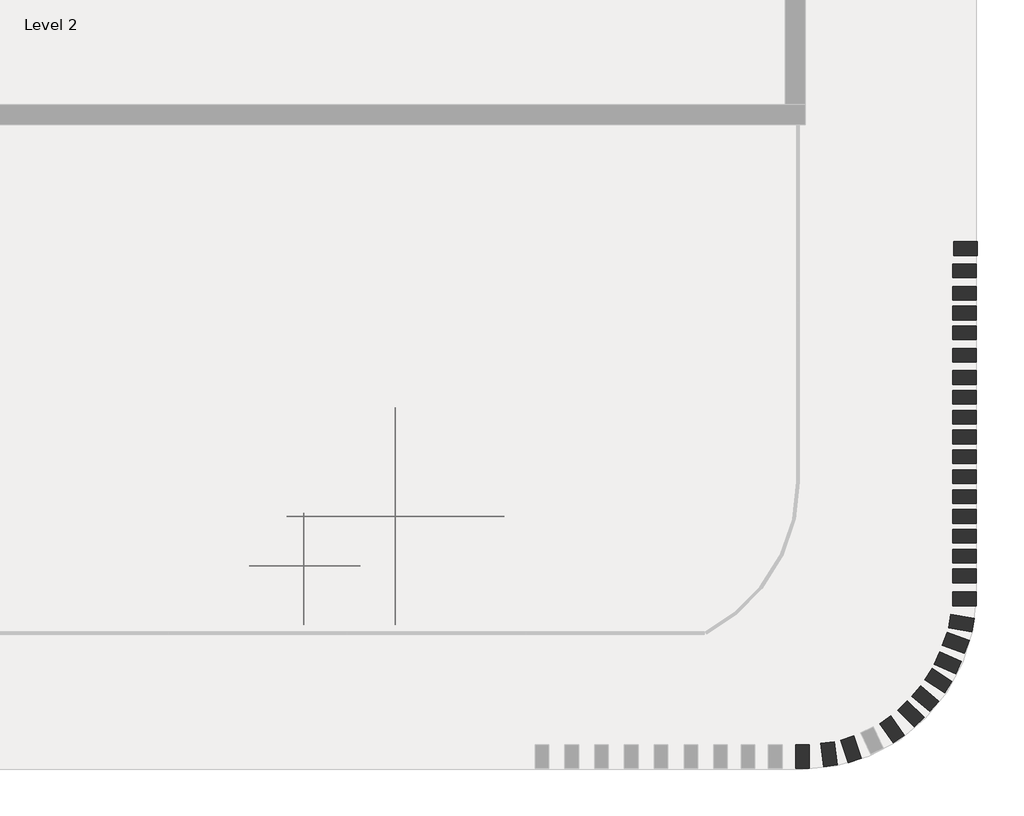
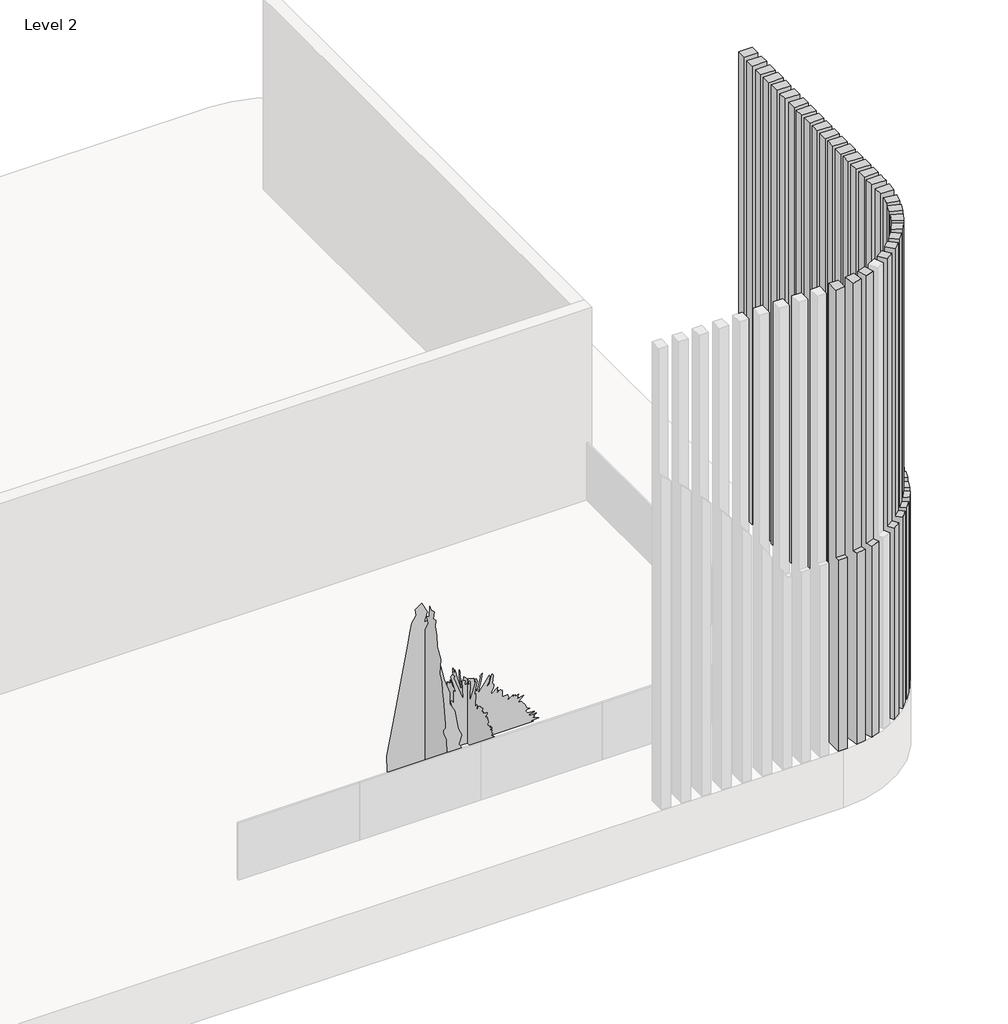
# One storey, part 2 of 2: 28 columns, 2 geographic elements.
"""IFC4 building model written with IfcOpenShell, lengths in millimetres."""

from ifc_helpers import new_model, si_unit, frame, origin, place, context, project, spatial, polyline, circle_curve, outline, extrude, transform, mapped, element, save
from ifc_brep_helpers import plane_surface, cylinder_surface, advanced_brep
from components import geographic_element_87ae7408, rpc_tree_conifer_red_cedar_10_b4f4fd19

model = new_model("IFC4")

# Units and contexts
model_context = context("Model", 3, world=origin())
ifc_project = project(units=[si_unit("LENGTHUNIT", "METRE", prefix="MILLI")], contexts=[model_context])

# Site, building, storey
site = spatial("IfcSite", under=ifc_project)
building = spatial("IfcBuilding", under=site)
storey = spatial("IfcBuildingStorey", under=building, Name="Level 2", Elevation=3048.0)

# Columns
placement = place(None, origin())
element("IfcColumn", 1, ObjectType="Wood Timber Column : 6 x 10", at=placement, inside=storey, context=model_context, shape_type="SweptSolid", body=[
    extrude(outline(polyline([(3962.4, 3820.0466756), (3962.4, 4061.3466756), (7013.3940217, 4061.3466756), (7013.3940217, 4023.2466756), (11277.6, 4023.2466756), (11277.6, 3820.0466756), (3962.4, 3820.0466756)])), frame((0.0, 2903.1292748, 0.0), z_axis=(0.0, 1.0, 0.0), x_axis=(0.0, 0.0, 1.0)), (0.0, 0.0, 1.0), 139.7),
])
element("IfcColumn", 2, ObjectType="Wood Timber Column : 6 x 10", at=placement, inside=storey, context=model_context, shape_type="SweptSolid", body=[
    extrude(outline(polyline([(3962.4, 3807.3466756), (3962.4, 4048.6466756), (7013.3940217, 4048.6466756), (7013.3940217, 4023.2466756), (11277.6, 4023.2466756), (11277.6, 3807.3466756), (3962.4, 3807.3466756)])), frame((0.0, 2674.5292748, 0.0), z_axis=(0.0, 1.0, 0.0), x_axis=(0.0, 0.0, 1.0)), (0.0, 0.0, 1.0), 139.7),
])
element("IfcColumn", 3, ObjectType="Wood Timber Column : 6 x 10", at=placement, inside=storey, context=model_context, shape_type="SweptSolid", body=[
    extrude(outline(polyline([(3962.4, 3807.3466756), (3962.4, 4048.6466756), (7013.3940217, 4048.6466756), (7013.3940217, 4023.2466756), (11277.6, 4023.2466756), (11277.6, 3807.3466756), (3962.4, 3807.3466756)])), frame((0.0, 2445.9292748, 0.0), z_axis=(0.0, 1.0, 0.0), x_axis=(0.0, 0.0, 1.0)), (0.0, 0.0, 1.0), 139.7),
])
element("IfcColumn", 4, ObjectType="Wood Timber Column : 6 x 10", at=placement, inside=storey, context=model_context, shape_type="SweptSolid", body=[
    extrude(outline(polyline([(3962.4, 3807.3466756), (3962.4, 4048.6466756), (7013.3940217, 4048.6466756), (7013.3940217, 4023.2466756), (11277.6, 4023.2466756), (11277.6, 3807.3466756), (3962.4, 3807.3466756)])), frame((0.0, 2242.7292748, 0.0), z_axis=(0.0, 1.0, 0.0), x_axis=(0.0, 0.0, 1.0)), (0.0, 0.0, 1.0), 139.7),
])
element("IfcColumn", 5, ObjectType="Wood Timber Column : 6 x 10", at=placement, inside=storey, context=model_context, shape_type="SweptSolid", body=[
    extrude(outline(polyline([(3962.4, 3807.3466756), (3962.4, 4048.6466756), (7013.3940217, 4048.6466756), (7013.3940217, 4023.2466756), (11277.6, 4023.2466756), (11277.6, 3807.3466756), (3962.4, 3807.3466756)])), frame((0.0, 2039.5292748, 0.0), z_axis=(0.0, 1.0, 0.0), x_axis=(0.0, 0.0, 1.0)), (0.0, 0.0, 1.0), 139.7),
])
element("IfcColumn", 6, ObjectType="Wood Timber Column : 6 x 10", at=placement, inside=storey, context=model_context, shape_type="SweptSolid", body=[
    extrude(outline(polyline([(3962.4, 3807.3466756), (3962.4, 4048.6466756), (7013.3940217, 4048.6466756), (7013.3940217, 4023.2466756), (11277.6, 4023.2466756), (11277.6, 3807.3466756), (3962.4, 3807.3466756)])), frame((0.0, 1810.9292748, 0.0), z_axis=(0.0, 1.0, 0.0), x_axis=(0.0, 0.0, 1.0)), (0.0, 0.0, 1.0), 139.7),
])
element("IfcColumn", 7, ObjectType="Wood Timber Column : 6 x 10", at=placement, inside=storey, context=model_context, shape_type="SweptSolid", body=[
    extrude(outline(polyline([(3962.4, 3807.3466756), (3962.4, 4048.6466756), (7013.3940217, 4048.6466756), (7013.3940217, 4023.2466756), (11277.6, 4023.2466756), (11277.6, 3807.3466756), (3962.4, 3807.3466756)])), frame((0.0, 1582.3292748, 0.0), z_axis=(0.0, 1.0, 0.0), x_axis=(0.0, 0.0, 1.0)), (0.0, 0.0, 1.0), 139.7),
])
element("IfcColumn", 8, ObjectType="Wood Timber Column : 6 x 10", at=placement, inside=storey, context=model_context, shape_type="SweptSolid", body=[
    extrude(outline(polyline([(3962.4, 3807.3466756), (3962.4, 4048.6466756), (7013.3940217, 4048.6466756), (7013.3940217, 4023.2466756), (11277.6, 4023.2466756), (11277.6, 3807.3466756), (3962.4, 3807.3466756)])), frame((0.0, 1379.1292748, 0.0), z_axis=(0.0, 1.0, 0.0), x_axis=(0.0, 0.0, 1.0)), (0.0, 0.0, 1.0), 139.7),
])
element("IfcColumn", 9, ObjectType="Wood Timber Column : 6 x 10", at=placement, inside=storey, context=model_context, shape_type="SweptSolid", body=[
    extrude(outline(polyline([(3962.4, 3807.3466756), (3962.4, 4048.6466756), (7013.3940217, 4048.6466756), (7013.3940217, 4023.2466756), (11277.6, 4023.2466756), (11277.6, 3807.3466756), (3962.4, 3807.3466756)])), frame((0.0, 1175.9292748, 0.0), z_axis=(0.0, 1.0, 0.0), x_axis=(0.0, 0.0, 1.0)), (0.0, 0.0, 1.0), 139.7),
])
element("IfcColumn", 10, ObjectType="Wood Timber Column : 6 x 10", at=placement, inside=storey, context=model_context, shape_type="SweptSolid", body=[
    extrude(outline(polyline([(3962.4, 3807.3466756), (3962.4, 4048.6466756), (7013.3940217, 4048.6466756), (7013.3940217, 4023.2466756), (11277.6, 4023.2466756), (11277.6, 3807.3466756), (3962.4, 3807.3466756)])), frame((0.0, 972.7292748, 0.0), z_axis=(0.0, 1.0, 0.0), x_axis=(0.0, 0.0, 1.0)), (0.0, 0.0, 1.0), 139.7),
])
element("IfcColumn", 11, ObjectType="Wood Timber Column : 6 x 10", at=placement, inside=storey, context=model_context, shape_type="SweptSolid", body=[
    extrude(outline(polyline([(3962.4, 3807.3466756), (3962.4, 4048.6466756), (7013.3940217, 4048.6466756), (7013.3940217, 4023.2466756), (11277.6, 4023.2466756), (11277.6, 3807.3466756), (3962.4, 3807.3466756)])), frame((0.0, 769.5292748, 0.0), z_axis=(0.0, 1.0, 0.0), x_axis=(0.0, 0.0, 1.0)), (0.0, 0.0, 1.0), 139.7),
])
element("IfcColumn", 12, ObjectType="Wood Timber Column : 6 x 10", at=placement, inside=storey, context=model_context, shape_type="SweptSolid", body=[
    extrude(outline(polyline([(3962.4, 3807.3466756), (3962.4, 4048.6466756), (7013.3940217, 4048.6466756), (7013.3940217, 4023.2466756), (11277.6, 4023.2466756), (11277.6, 3807.3466756), (3962.4, 3807.3466756)])), frame((0.0, 566.3292748, 0.0), z_axis=(0.0, 1.0, 0.0), x_axis=(0.0, 0.0, 1.0)), (0.0, 0.0, 1.0), 139.7),
])
element("IfcColumn", 13, ObjectType="Wood Timber Column : 6 x 10", at=placement, inside=storey, context=model_context, shape_type="SweptSolid", body=[
    extrude(outline(polyline([(3962.4, 3807.3466756), (3962.4, 4048.6466756), (7013.3940217, 4048.6466756), (7013.3940217, 4023.2466756), (11277.6, 4023.2466756), (11277.6, 3807.3466756), (3962.4, 3807.3466756)])), frame((0.0, 363.1292748, 0.0), z_axis=(0.0, 1.0, 0.0), x_axis=(0.0, 0.0, 1.0)), (0.0, 0.0, 1.0), 139.7),
])
element("IfcColumn", 14, ObjectType="Wood Timber Column : 6 x 10", at=placement, inside=storey, context=model_context, shape_type="SweptSolid", body=[
    extrude(outline(polyline([(3962.4, 3807.3466756), (3962.4, 4048.6466756), (7013.3940217, 4048.6466756), (7013.3940217, 4023.2466756), (11277.6, 4023.2466756), (11277.6, 3807.3466756), (3962.4, 3807.3466756)])), frame((0.0, 159.9292748, 0.0), z_axis=(0.0, 1.0, 0.0), x_axis=(0.0, 0.0, 1.0)), (0.0, 0.0, 1.0), 139.7),
])
element("IfcColumn", 15, ObjectType="Wood Timber Column : 6 x 10", at=placement, inside=storey, context=model_context, shape_type="SweptSolid", body=[
    extrude(outline(polyline([(3962.4, 3807.3466756), (3962.4, 4048.6466756), (7013.3940217, 4048.6466756), (7013.3940217, 4023.2466756), (11277.6, 4023.2466756), (11277.6, 3807.3466756), (3962.4, 3807.3466756)])), frame((0.0, -43.2707252, 0.0), z_axis=(0.0, 1.0, 0.0), x_axis=(0.0, 0.0, 1.0)), (0.0, 0.0, 1.0), 139.7),
])
element("IfcColumn", 16, ObjectType="Wood Timber Column : 6 x 10", at=placement, inside=storey, context=model_context, shape_type="SweptSolid", body=[
    extrude(outline(polyline([(3962.4, 3807.3466756), (3962.4, 4048.6466756), (7013.3940217, 4048.6466756), (7013.3940217, 4023.2466756), (11277.6, 4023.2466756), (11277.6, 3807.3466756), (3962.4, 3807.3466756)])), frame((0.0, -246.4707252, 0.0), z_axis=(0.0, 1.0, 0.0), x_axis=(0.0, 0.0, 1.0)), (0.0, 0.0, 1.0), 139.7),
])
element("IfcColumn", 17, ObjectType="Wood Timber Column : 6 x 10", at=placement, inside=storey, context=model_context, shape_type="AdvancedBrep", body=[
    advanced_brep(
    [(4048.6466756, -309.9707252, 3962.4), (4048.6466756, -449.6707252, 3962.4), (3807.3466756, -449.6707252, 3962.4), (3807.3466756, -309.9707252, 3962.4), (4048.6466756, -309.9707252, 7013.3940217), (4048.6466756, -405.3567338, 7013.3940217), (4048.6466756, -405.3567338, 7010.4), (4048.6466756, -449.6707252, 7010.4), (4022.7274738, -449.6707252, 7010.4), (4022.7274738, -449.6707252, 11277.6), (3807.3466756, -449.6707252, 11277.6), (3807.3466756, -309.9707252, 11277.6), (4023.2466756, -309.9707252, 11277.6), (4023.2466756, -309.9707252, 7013.3940217), (4023.2466756, -405.3567338, 11277.6), (4023.2466756, -405.3567338, 7013.3940217), (4023.2466756, -405.3567338, 7010.4)],
    [
        (0, 1),
        (1, 2),
        (2, 3),
        (3, 0),
        (0, 4),
        (4, 5),
        (5, 6),
        (6, 7),
        (7, 1),
        (7, 8),
        (8, 9),
        (9, 10),
        (10, 2),
        (10, 11),
        (11, 3),
        (11, 12),
        (12, 13),
        (13, 4),
        (9, 14, circle_curve(frame((2131.8825083, -405.3567338, 11277.6), z_axis=(0.0, 0.0, 1.0), x_axis=(1.0, 0.0, 0.0)), 1891.3641672)),
        (14, 12),
        (13, 15),
        (15, 5),
        (14, 15),
        (6, 16),
        (16, 8, circle_curve(frame((2131.8825083, -405.3567338, 7010.4), z_axis=(0.0, 0.0, -1.0), x_axis=(1.0, 0.0, 0.0)), 1891.3641672)),
        (15, 16),
    ],
    [
        plane_surface(frame((4048.6466756, -309.9707252, 3962.4), z_axis=(0.0, 0.0, -1.0), x_axis=(1.0, 0.0, 0.0))),
        plane_surface(frame((4048.6466756, -449.6707252, 11277.6), z_axis=(1.0, 0.0, 0.0), x_axis=(0.0, 0.0, -1.0))),
        plane_surface(frame((3807.3466756, -449.6707252, 11277.6), z_axis=(0.0, -1.0, 0.0), x_axis=(0.0, 0.0, -1.0))),
        plane_surface(frame((3807.3466756, -309.9707252, 11277.6), z_axis=(-1.0, 0.0, 0.0), x_axis=(0.0, 0.0, -1.0))),
        plane_surface(frame((4048.6466756, -309.9707252, 11277.6), z_axis=(0.0, 1.0, 0.0), x_axis=(0.0, 0.0, -1.0))),
        plane_surface(frame((4048.6466756, -309.9707252, 11277.6), z_axis=(0.0, 0.0, 1.0), x_axis=(-1.0, 0.0, 0.0))),
        plane_surface(frame((4226.4466756, -405.3567338, 7013.3940217), z_axis=(0.0, 0.0, 1.0), x_axis=(-1.0, 0.0, 0.0))),
        plane_surface(frame((4023.2466756, 661.4432662, 7013.3940217), z_axis=(1.0, 0.0, 0.0), x_axis=(0.0, -1.0, 0.0))),
        plane_surface(frame((4226.4466756, -405.3567338, 7010.4), z_axis=(0.0, 0.0, 1.0), x_axis=(0.0, -1.0, 0.0))),
        plane_surface(frame((4226.4466756, -405.3567338, 11893.55), z_axis=(0.0, -1.0, 0.0), x_axis=(0.0, 0.0, -1.0))),
        cylinder_surface(frame((2131.8825083, -405.3567338, 7010.4), z_axis=(0.0, 0.0, -1.0), x_axis=(1.0, 0.0, 0.0)), 1891.3641672),
    ],
    [
        (0, [[1, 2, 3, 4]]),
        (1, [[-1, 5, 6, 7, 8, 9]]),
        (2, [[-2, -9, 10, 11, 12, 13]]),
        (3, [[-3, -13, 14, 15]]),
        (4, [[-4, -15, 16, 17, 18, -5]]),
        (5, [[-14, -12, 19, 20, -16]]),
        (6, [[-18, 21, 22, -6]]),
        (7, [[-21, -17, -20, 23]]),
        (8, [[24, 25, -10, -8]]),
        (9, [[26, -24, -7, -22]]),
        (10, [[-26, -23, -19, -11, -25]]),
    ],
),
])
element("IfcColumn", 18, ObjectType="Wood Timber Column : 6 x 10", at=placement, inside=storey, context=model_context, shape_type="AdvancedBrep", body=[
    advanced_brep(
    [(4048.6466756, -545.0567338, 3962.4), (4048.6466756, -684.7567338, 3962.4), (3807.3466756, -684.7567338, 3962.4), (3807.3466756, -545.0567338, 3962.4), (4048.6466756, -545.0567338, 7010.4), (4048.6466756, -684.7567338, 7010.4), (4002.4957909, -684.7567338, 7010.4), (4002.4957909, -684.7567338, 11277.6), (3807.3466756, -684.7567338, 11277.6), (3807.3466756, -545.0567338, 11277.6), (4018.0803567, -545.0567338, 11277.6), (4018.0803567, -545.0567338, 7010.4)],
    [
        (0, 1),
        (1, 2),
        (2, 3),
        (3, 0),
        (0, 4),
        (4, 5),
        (5, 1),
        (5, 6),
        (6, 7),
        (7, 8),
        (8, 2),
        (8, 9),
        (9, 3),
        (9, 10),
        (10, 11),
        (11, 4),
        (7, 10, circle_curve(frame((2131.8825083, -405.3567338, 11277.6), z_axis=(0.0, 0.0, 1.0), x_axis=(1.0, 0.0, 0.0)), 1891.3641672)),
        (11, 6, circle_curve(frame((2131.8825083, -405.3567338, 7010.4), z_axis=(0.0, 0.0, -1.0), x_axis=(1.0, 0.0, 0.0)), 1891.3641672)),
    ],
    [
        plane_surface(frame((4048.6466756, -545.0567338, 3962.4), z_axis=(0.0, 0.0, -1.0), x_axis=(1.0, 0.0, 0.0))),
        plane_surface(frame((4048.6466756, -684.7567338, 11277.6), z_axis=(1.0, 0.0, 0.0), x_axis=(0.0, 0.0, -1.0))),
        plane_surface(frame((3807.3466756, -684.7567338, 11277.6), z_axis=(0.0, -1.0, 0.0), x_axis=(0.0, 0.0, -1.0))),
        plane_surface(frame((3807.3466756, -545.0567338, 11277.6), z_axis=(-1.0, 0.0, 0.0), x_axis=(0.0, 0.0, -1.0))),
        plane_surface(frame((4048.6466756, -545.0567338, 11277.6), z_axis=(0.0, 1.0, 0.0), x_axis=(0.0, 0.0, -1.0))),
        plane_surface(frame((4048.6466756, -545.0567338, 11277.6), z_axis=(0.0, 0.0, 1.0), x_axis=(-1.0, 0.0, 0.0))),
        plane_surface(frame((4226.4466756, -405.3567338, 7010.4), z_axis=(0.0, 0.0, 1.0), x_axis=(0.0, -1.0, 0.0))),
        cylinder_surface(frame((2131.8825083, -405.3567338, 7010.4), z_axis=(0.0, 0.0, -1.0), x_axis=(1.0, 0.0, 0.0)), 1891.3641672),
    ],
    [
        (0, [[1, 2, 3, 4]]),
        (1, [[-1, 5, 6, 7]]),
        (2, [[-2, -7, 8, 9, 10, 11]]),
        (3, [[-3, -11, 12, 13]]),
        (4, [[-4, -13, 14, 15, 16, -5]]),
        (5, [[-12, -10, 17, -14]]),
        (6, [[18, -8, -6, -16]]),
        (7, [[-18, -15, -17, -9]]),
    ],
),
])
element("IfcColumn", 19, ObjectType="Wood Timber Column : 6 x 10", at=placement, inside=storey, context=model_context, shape_type="AdvancedBrep", body=[
    advanced_brep(
    [(4027.1930562, -814.7185649, 3962.4), (4002.9344058, -952.296208, 3962.4), (3765.300295, -910.3949027, 3962.4), (3789.5589454, -772.8172596, 3962.4), (4027.1930562, -814.7185649, 7010.4), (4002.9344058, -952.296208, 7010.4), (3945.4692461, -942.1635499, 7010.4), (3945.4692461, -942.1635499, 11277.6), (3765.300295, -910.3949027, 11277.6), (3789.5589454, -772.8172596, 11277.6), (3980.2310455, -806.4378953, 11277.6), (3980.2310455, -806.4378953, 7010.4)],
    [
        (0, 1),
        (1, 2),
        (2, 3),
        (3, 0),
        (0, 4),
        (4, 5),
        (5, 1),
        (5, 6),
        (6, 7),
        (7, 8),
        (8, 2),
        (8, 9),
        (9, 3),
        (9, 10),
        (10, 11),
        (11, 4),
        (7, 10, circle_curve(frame((2131.8825083, -405.3567338, 11277.6), z_axis=(0.0, 0.0, 1.0), x_axis=(1.0, 0.0, 0.0)), 1891.3641672)),
        (11, 6, circle_curve(frame((2131.8825083, -405.3567338, 7010.4), z_axis=(0.0, 0.0, -1.0), x_axis=(1.0, 0.0, 0.0)), 1891.3641672)),
    ],
    [
        plane_surface(frame((4027.1930562, -814.7185649, 3962.4), z_axis=(0.0, 0.0, -1.0), x_axis=(0.9848077530122077, -0.1736481776669326, 0.0))),
        plane_surface(frame((4002.9344058, -952.296208, 11277.6), z_axis=(0.9848077530122077, -0.1736481776669326, 0.0), x_axis=(0.0, 0.0, -1.0))),
        plane_surface(frame((3765.300295, -910.3949027, 11277.6), z_axis=(-0.1736481776669326, -0.9848077530122077, 0.0), x_axis=(0.0, 0.0, -1.0))),
        plane_surface(frame((3789.5589454, -772.8172596, 11277.6), z_axis=(-0.9848077530122077, 0.1736481776669326, 0.0), x_axis=(0.0, 0.0, -1.0))),
        plane_surface(frame((4027.1930562, -814.7185649, 11277.6), z_axis=(0.1736481776669326, 0.9848077530122077, 0.0), x_axis=(0.0, 0.0, -1.0))),
        plane_surface(frame((4027.1930562, -814.7185649, 11277.6), z_axis=(0.0, 0.0, 1.0), x_axis=(-0.9848077530122077, 0.1736481776669326, 0.0))),
        plane_surface(frame((4226.4466756, -405.3567338, 7010.4), z_axis=(0.0, 0.0, 1.0), x_axis=(0.0, -1.0, 0.0))),
        cylinder_surface(frame((2131.8825083, -405.3567338, 7010.4), z_axis=(0.0, 0.0, -1.0), x_axis=(1.0, 0.0, 0.0)), 1891.3641672),
    ],
    [
        (0, [[1, 2, 3, 4]]),
        (1, [[-1, 5, 6, 7]]),
        (2, [[-2, -7, 8, 9, 10, 11]]),
        (3, [[-3, -11, 12, 13]]),
        (4, [[-4, -13, 14, 15, 16, -5]]),
        (5, [[-12, -10, 17, -14]]),
        (6, [[18, -8, -6, -16]]),
        (7, [[-18, -15, -17, -9]]),
    ],
),
])
element("IfcColumn", 20, ObjectType="Wood Timber Column : 6 x 10", at=placement, inside=storey, context=model_context, shape_type="AdvancedBrep", body=[
    advanced_brep(
    [(3976.3606973, -1041.3839345, 3962.4), (3928.5804832, -1172.6589937, 3962.4), (3701.8326539, -1090.1295331, 3962.4), (3749.6128679, -958.8544739, 3962.4), (3976.3606973, -1041.3839345, 7010.4), (3928.5804832, -1172.6589937, 7010.4), (3869.9300311, -1151.3119749, 7010.4), (3869.9300311, -1151.3119749, 11277.6), (3701.8326539, -1090.1295331, 11277.6), (3749.6128679, -958.8544739, 11277.6), (3920.257735, -1020.9641262, 11277.6), (3920.257735, -1020.9641262, 7010.4)],
    [
        (0, 1),
        (1, 2),
        (2, 3),
        (3, 0),
        (0, 4),
        (4, 5),
        (5, 1),
        (5, 6),
        (6, 7),
        (7, 8),
        (8, 2),
        (8, 9),
        (9, 3),
        (9, 10),
        (10, 11),
        (11, 4),
        (7, 10, circle_curve(frame((2131.8825083, -405.3567338, 11277.6), z_axis=(0.0, 0.0, 1.0), x_axis=(1.0, 0.0, 0.0)), 1891.3641672)),
        (11, 6, circle_curve(frame((2131.8825083, -405.3567338, 7010.4), z_axis=(0.0, 0.0, -1.0), x_axis=(1.0, 0.0, 0.0)), 1891.3641672)),
    ],
    [
        plane_surface(frame((3976.3606973, -1041.3839345, 3962.4), z_axis=(0.0, 0.0, -1.0), x_axis=(0.9396926207859073, -0.3420201433256717, 0.0))),
        plane_surface(frame((3928.5804832, -1172.6589937, 11277.6), z_axis=(0.9396926207859073, -0.3420201433256717, 0.0), x_axis=(0.0, 0.0, -1.0))),
        plane_surface(frame((3701.8326539, -1090.1295331, 11277.6), z_axis=(-0.3420201433256717, -0.9396926207859073, 0.0), x_axis=(0.0, 0.0, -1.0))),
        plane_surface(frame((3749.6128679, -958.8544739, 11277.6), z_axis=(-0.9396926207859073, 0.3420201433256717, 0.0), x_axis=(0.0, 0.0, -1.0))),
        plane_surface(frame((3976.3606973, -1041.3839345, 11277.6), z_axis=(0.3420201433256717, 0.9396926207859073, 0.0), x_axis=(0.0, 0.0, -1.0))),
        plane_surface(frame((3976.3606973, -1041.3839345, 11277.6), z_axis=(0.0, 0.0, 1.0), x_axis=(-0.9396926207859073, 0.3420201433256717, 0.0))),
        plane_surface(frame((4226.4466756, -405.3567338, 7010.4), z_axis=(0.0, 0.0, 1.0), x_axis=(0.0, -1.0, 0.0))),
        cylinder_surface(frame((2131.8825083, -405.3567338, 7010.4), z_axis=(0.0, 0.0, -1.0), x_axis=(1.0, 0.0, 0.0)), 1891.3641672),
    ],
    [
        (0, [[1, 2, 3, 4]]),
        (1, [[-1, 5, 6, 7]]),
        (2, [[-2, -7, 8, 9, 10, 11]]),
        (3, [[-3, -11, 12, 13]]),
        (4, [[-4, -13, 14, 15, 16, -5]]),
        (5, [[-12, -10, 17, -14]]),
        (6, [[18, -8, -6, -16]]),
        (7, [[-18, -15, -17, -9]]),
    ],
),
])
element("IfcColumn", 21, ObjectType="Wood Timber Column : 6 x 10", at=placement, inside=storey, context=model_context, shape_type="AdvancedBrep", body=[
    advanced_brep(
    [(3895.1919816, -1254.3648146, 3962.4), (3838.2360857, -1381.9270187, 3962.4), (3617.9013695, -1283.548653, 3962.4), (3674.8572654, -1155.9864489, 3962.4), (3895.1919816, -1254.3648146, 7010.4), (3838.2360857, -1381.9270187, 7010.4), (3769.6889417, -1351.3210565, 7010.4), (3769.6889417, -1351.3210565, 11277.6), (3617.9013695, -1283.548653, 11277.6), (3674.8572654, -1155.9864489, 11277.6), (3835.1804364, -1227.5699552, 11277.6), (3835.1804364, -1227.5699552, 7010.4)],
    [
        (0, 1),
        (1, 2),
        (2, 3),
        (3, 0),
        (0, 4),
        (4, 5),
        (5, 1),
        (5, 6),
        (6, 7),
        (7, 8),
        (8, 2),
        (8, 9),
        (9, 3),
        (9, 10),
        (10, 11),
        (11, 4),
        (7, 10, circle_curve(frame((2131.8825083, -405.3567338, 11277.6), z_axis=(0.0, 0.0, 1.0), x_axis=(1.0, 0.0, 0.0)), 1891.3641672)),
        (11, 6, circle_curve(frame((2131.8825083, -405.3567338, 7010.4), z_axis=(0.0, 0.0, -1.0), x_axis=(1.0, 0.0, 0.0)), 1891.3641672)),
    ],
    [
        plane_surface(frame((3895.1919816, -1254.3648146, 3962.4), z_axis=(0.0, 0.0, -1.0), x_axis=(0.9131152763933513, -0.40770147414142816, 0.0))),
        plane_surface(frame((3838.2360857, -1381.9270187, 11277.6), z_axis=(0.9131152763933513, -0.40770147414142816, 0.0), x_axis=(0.0, 0.0, -1.0))),
        plane_surface(frame((3617.9013695, -1283.548653, 11277.6), z_axis=(-0.40770147414142816, -0.9131152763933513, 0.0), x_axis=(0.0, 0.0, -1.0))),
        plane_surface(frame((3674.8572654, -1155.9864489, 11277.6), z_axis=(-0.9131152763933513, 0.40770147414142816, 0.0), x_axis=(0.0, 0.0, -1.0))),
        plane_surface(frame((3895.1919816, -1254.3648146, 11277.6), z_axis=(0.40770147414142816, 0.9131152763933513, 0.0), x_axis=(0.0, 0.0, -1.0))),
        plane_surface(frame((3895.1919816, -1254.3648146, 11277.6), z_axis=(0.0, 0.0, 1.0), x_axis=(-0.9131152763933513, 0.40770147414142816, 0.0))),
        plane_surface(frame((4226.4466756, -405.3567338, 7010.4), z_axis=(0.0, 0.0, 1.0), x_axis=(0.0, -1.0, 0.0))),
        cylinder_surface(frame((2131.8825083, -405.3567338, 7010.4), z_axis=(0.0, 0.0, -1.0), x_axis=(1.0, 0.0, 0.0)), 1891.3641672),
    ],
    [
        (0, [[1, 2, 3, 4]]),
        (1, [[-1, 5, 6, 7]]),
        (2, [[-2, -7, 8, 9, 10, 11]]),
        (3, [[-3, -11, 12, 13]]),
        (4, [[-4, -13, 14, 15, 16, -5]]),
        (5, [[-12, -10, 17, -14]]),
        (6, [[18, -8, -6, -16]]),
        (7, [[-18, -15, -17, -9]]),
    ],
),
])
element("IfcColumn", 22, ObjectType="Wood Timber Column : 6 x 10", at=placement, inside=storey, context=model_context, shape_type="AdvancedBrep", body=[
    advanced_brep(
    [(3800.5253162, -1460.2362942, 3962.4), (3724.439243, -1577.3985725, 3962.4), (3522.0680349, -1445.9771734, 3962.4), (3598.1541081, -1328.8148951, 3962.4), (3800.5253162, -1460.2362942, 7010.4), (3724.439243, -1577.3985725, 7010.4), (3652.1950217, -1530.4826267, 7010.4), (3652.1950217, -1530.4826267, 11277.6), (3522.0680349, -1445.9771734, 11277.6), (3598.1541081, -1328.8148951, 11277.6), (3731.1171696, -1415.1621168, 11277.6), (3731.1171696, -1415.1621168, 7010.4)],
    [
        (0, 1),
        (1, 2),
        (2, 3),
        (3, 0),
        (0, 4),
        (4, 5),
        (5, 1),
        (5, 6),
        (6, 7),
        (7, 8),
        (8, 2),
        (8, 9),
        (9, 3),
        (9, 10),
        (10, 11),
        (11, 4),
        (7, 10, circle_curve(frame((2131.8825083, -405.3567338, 11277.6), z_axis=(0.0, 0.0, 1.0), x_axis=(1.0, 0.0, 0.0)), 1891.3641672)),
        (11, 6, circle_curve(frame((2131.8825083, -405.3567338, 7010.4), z_axis=(0.0, 0.0, -1.0), x_axis=(1.0, 0.0, 0.0)), 1891.3641672)),
    ],
    [
        plane_surface(frame((3800.5253162, -1460.2362942, 3962.4), z_axis=(0.0, 0.0, -1.0000000000000002), x_axis=(0.8386705679454228, -0.5446390350150291, 0.0))),
        plane_surface(frame((3724.439243, -1577.3985725, 11277.6), z_axis=(0.8386705679454228, -0.5446390350150291, 0.0), x_axis=(0.0, 0.0, -1.0))),
        plane_surface(frame((3522.0680349, -1445.9771734, 11277.6), z_axis=(-0.5446390350150291, -0.8386705679454228, 0.0), x_axis=(0.0, 0.0, -1.0))),
        plane_surface(frame((3598.1541081, -1328.8148951, 11277.6), z_axis=(-0.8386705679454228, 0.5446390350150291, 0.0), x_axis=(0.0, 0.0, -1.0))),
        plane_surface(frame((3800.5253162, -1460.2362942, 11277.6), z_axis=(0.5446390350150291, 0.8386705679454228, 0.0), x_axis=(0.0, 0.0, -1.0))),
        plane_surface(frame((3800.5253162, -1460.2362942, 11277.6), z_axis=(0.0, 0.0, 1.0000000000000002), x_axis=(-0.8386705679454228, 0.5446390350150291, 0.0))),
        plane_surface(frame((4226.4466756, -405.3567338, 7010.4), z_axis=(0.0, 0.0, 1.0), x_axis=(0.0, -1.0, 0.0))),
        cylinder_surface(frame((2131.8825083, -405.3567338, 7010.4), z_axis=(0.0, 0.0, -1.0), x_axis=(1.0, 0.0, 0.0)), 1891.3641672),
    ],
    [
        (0, [[1, 2, 3, 4]]),
        (1, [[-1, 5, 6, 7]]),
        (2, [[-2, -7, 8, 9, 10, 11]]),
        (3, [[-3, -11, 12, 13]]),
        (4, [[-4, -13, 14, 15, 16, -5]]),
        (5, [[-12, -10, 17, -14]]),
        (6, [[18, -8, -6, -16]]),
        (7, [[-18, -15, -17, -9]]),
    ],
),
])
element("IfcColumn", 23, ObjectType="Wood Timber Column : 6 x 10", at=placement, inside=storey, context=model_context, shape_type="AdvancedBrep", body=[
    advanced_brep(
    [(3665.1125252, -1662.1760976, 3962.4), (3574.6344553, -1768.6176725, 3962.4), (3390.7808259, -1612.33737, 3962.4), (3481.2588958, -1505.8957951, 3962.4), (3665.1125252, -1662.1760976, 7010.4), (3574.6344553, -1768.6176725, 7010.4), (3503.2275911, -1707.9200057, 7010.4), (3503.2275911, -1707.9200057, 11277.6), (3390.7808259, -1612.33737, 11277.6), (3481.2588958, -1505.8957951, 11277.6), (3595.6458794, -1603.1276662, 11277.6), (3595.6458794, -1603.1276662, 7010.4)],
    [
        (0, 1),
        (1, 2),
        (2, 3),
        (3, 0),
        (0, 4),
        (4, 5),
        (5, 1),
        (5, 6),
        (6, 7),
        (7, 8),
        (8, 2),
        (8, 9),
        (9, 3),
        (9, 10),
        (10, 11),
        (11, 4),
        (7, 10, circle_curve(frame((2131.8825083, -405.3567338, 11277.6), z_axis=(0.0, 0.0, 1.0), x_axis=(1.0, 0.0, 0.0)), 1891.3641672)),
        (11, 6, circle_curve(frame((2131.8825083, -405.3567338, 7010.4), z_axis=(0.0, 0.0, -1.0), x_axis=(1.0, 0.0, 0.0)), 1891.3641672)),
    ],
    [
        plane_surface(frame((3665.1125252, -1662.1760976, 3962.4), z_axis=(0.0, 0.0, -1.0), x_axis=(0.7619296699862876, -0.6476597702456026, 0.0))),
        plane_surface(frame((3574.6344553, -1768.6176725, 11277.6), z_axis=(0.7619296699862876, -0.6476597702456026, 0.0), x_axis=(0.0, 0.0, -1.0))),
        plane_surface(frame((3390.7808259, -1612.33737, 11277.6), z_axis=(-0.6476597702456026, -0.7619296699862876, 0.0), x_axis=(0.0, 0.0, -1.0))),
        plane_surface(frame((3481.2588958, -1505.8957951, 11277.6), z_axis=(-0.7619296699862876, 0.6476597702456026, 0.0), x_axis=(0.0, 0.0, -1.0))),
        plane_surface(frame((3665.1125252, -1662.1760976, 11277.6), z_axis=(0.6476597702456026, 0.7619296699862876, 0.0), x_axis=(0.0, 0.0, -1.0))),
        plane_surface(frame((3665.1125252, -1662.1760976, 11277.6), z_axis=(0.0, 0.0, 1.0), x_axis=(-0.7619296699862876, 0.6476597702456026, 0.0))),
        plane_surface(frame((4226.4466756, -405.3567338, 7010.4), z_axis=(0.0, 0.0, 1.0), x_axis=(0.0, -1.0, 0.0))),
        cylinder_surface(frame((2131.8825083, -405.3567338, 7010.4), z_axis=(0.0, 0.0, -1.0), x_axis=(1.0, 0.0, 0.0)), 1891.3641672),
    ],
    [
        (0, [[1, 2, 3, 4]]),
        (1, [[-1, 5, 6, 7]]),
        (2, [[-2, -7, 8, 9, 10, 11]]),
        (3, [[-3, -11, 12, 13]]),
        (4, [[-4, -13, 14, 15, 16, -5]]),
        (5, [[-12, -10, 17, -14]]),
        (6, [[18, -8, -6, -16]]),
        (7, [[-18, -15, -17, -9]]),
    ],
),
])
element("IfcColumn", 24, ObjectType="Wood Timber Column : 6 x 10", at=placement, inside=storey, context=model_context, shape_type="AdvancedBrep", body=[
    advanced_brep(
    [(3515.355698, -1828.8208207, 3962.4), (3416.5728806, -1927.603638, 3962.4), (3245.9480143, -1756.9787717, 3962.4), (3344.7308317, -1658.1959544, 3962.4), (3515.355698, -1828.8208207, 7010.4), (3416.5728806, -1927.603638, 7010.4), (3345.215698, -1856.2464553, 7010.4), (3345.215698, -1856.2464553, 11277.6), (3245.9480143, -1756.9787717, 11277.6), (3344.7308317, -1658.1959544, 11277.6), (3449.1340035, -1762.5991262, 11277.6), (3449.1340035, -1762.5991262, 7010.4)],
    [
        (0, 1),
        (1, 2),
        (2, 3),
        (3, 0),
        (0, 4),
        (4, 5),
        (5, 1),
        (5, 6),
        (6, 7),
        (7, 8),
        (8, 2),
        (8, 9),
        (9, 3),
        (9, 10),
        (10, 11),
        (11, 4),
        (7, 10, circle_curve(frame((2131.8825083, -405.3567338, 11277.6), z_axis=(0.0, 0.0, 1.0), x_axis=(1.0, 0.0, 0.0)), 1891.3641672)),
        (11, 6, circle_curve(frame((2131.8825083, -405.3567338, 7010.4), z_axis=(0.0, 0.0, -1.0), x_axis=(1.0, 0.0, 0.0)), 1891.3641672)),
    ],
    [
        plane_surface(frame((3515.355698, -1828.8208207, 3962.4), z_axis=(0.0, 0.0, -1.0), x_axis=(0.7071067811865477, -0.7071067811865475, 0.0))),
        plane_surface(frame((3416.5728806, -1927.603638, 11277.6), z_axis=(0.7071067811865477, -0.7071067811865475, 0.0), x_axis=(0.0, 0.0, -1.0))),
        plane_surface(frame((3245.9480143, -1756.9787717, 11277.6), z_axis=(-0.7071067811865475, -0.7071067811865477, 0.0), x_axis=(0.0, 0.0, -1.0))),
        plane_surface(frame((3344.7308317, -1658.1959544, 11277.6), z_axis=(-0.7071067811865477, 0.7071067811865475, 0.0), x_axis=(0.0, 0.0, -1.0))),
        plane_surface(frame((3515.355698, -1828.8208207, 11277.6), z_axis=(0.7071067811865475, 0.7071067811865477, 0.0), x_axis=(0.0, 0.0, -1.0))),
        plane_surface(frame((3515.355698, -1828.8208207, 11277.6), z_axis=(0.0, 0.0, 1.0), x_axis=(-0.7071067811865477, 0.7071067811865475, 0.0))),
        plane_surface(frame((4226.4466756, -405.3567338, 7010.4), z_axis=(0.0, 0.0, 1.0), x_axis=(0.0, -1.0, 0.0))),
        cylinder_surface(frame((2131.8825083, -405.3567338, 7010.4), z_axis=(0.0, 0.0, -1.0), x_axis=(1.0, 0.0, 0.0)), 1891.3641672),
    ],
    [
        (0, [[1, 2, 3, 4]]),
        (1, [[-1, 5, 6, 7]]),
        (2, [[-2, -7, 8, 9, 10, 11]]),
        (3, [[-3, -11, 12, 13]]),
        (4, [[-4, -13, 14, 15, 16, -5]]),
        (5, [[-12, -10, 17, -14]]),
        (6, [[18, -8, -6, -16]]),
        (7, [[-18, -15, -17, -9]]),
    ],
),
])
element("IfcColumn", 25, ObjectType="Wood Timber Column : 6 x 10", at=placement, inside=storey, context=model_context, shape_type="AdvancedBrep", body=[
    advanced_brep(
    [(3058.6269082, -1892.8834161, 3962.4), (3173.0624488, -1812.754788, 3962.4), (3311.4664429, -2010.4161763, 3962.4), (3197.0309023, -2090.5448044, 3962.4), (3058.6269082, -1892.8834161, 11277.6), (3173.0624488, -1812.754788, 11277.6), (3253.7900559, -1928.0457591, 11277.6), (3253.7900559, -1928.0457591, 7010.4), (3311.4664429, -2010.4161763, 7010.4), (3197.0309023, -2090.5448044, 7010.4), (3138.3278205, -2006.7081152, 7010.4), (3138.3278205, -2006.7081152, 11277.6)],
    [
        (0, 1),
        (1, 2),
        (2, 3),
        (3, 0),
        (0, 4),
        (4, 5),
        (5, 1),
        (5, 6),
        (6, 7),
        (7, 8),
        (8, 2),
        (8, 9),
        (9, 3),
        (9, 10),
        (10, 11),
        (11, 4),
        (11, 6, circle_curve(frame((2131.8825083, -405.3567338, 11277.6), z_axis=(0.0, 0.0, 1.0), x_axis=(1.0, 0.0, 0.0)), 1891.3641672)),
        (7, 10, circle_curve(frame((2131.8825083, -405.3567338, 7010.4), z_axis=(0.0, 0.0, -1.0), x_axis=(1.0, 0.0, 0.0)), 1891.3641672)),
    ],
    [
        plane_surface(frame((3058.6269082, -1892.8834161, 3962.4), z_axis=(0.0, 0.0, -1.0000000000000002), x_axis=(-0.5735764363510424, 0.8191520442889945, 0.0))),
        plane_surface(frame((3173.0624488, -1812.754788, 11277.6), z_axis=(-0.5735764363510424, 0.8191520442889945, 0.0), x_axis=(0.0, 0.0, -1.0))),
        plane_surface(frame((3311.4664429, -2010.4161763, 11277.6), z_axis=(0.8191520442889945, 0.5735764363510424, 0.0), x_axis=(0.0, 0.0, -1.0))),
        plane_surface(frame((3197.0309023, -2090.5448044, 11277.6), z_axis=(0.5735764363510424, -0.8191520442889945, 0.0), x_axis=(0.0, 0.0, -1.0))),
        plane_surface(frame((3058.6269082, -1892.8834161, 11277.6), z_axis=(-0.8191520442889945, -0.5735764363510424, 0.0), x_axis=(0.0, 0.0, -1.0))),
        plane_surface(frame((3058.6269082, -1892.8834161, 11277.6), z_axis=(0.0, 0.0, 1.0000000000000002), x_axis=(0.5735764363510424, -0.8191520442889945, 0.0))),
        plane_surface(frame((4226.4466756, -405.3567338, 7010.4), z_axis=(0.0, 0.0, 1.0), x_axis=(0.0, -1.0, 0.0))),
        cylinder_surface(frame((2131.8825083, -405.3567338, 7010.4), z_axis=(0.0, 0.0, -1.0), x_axis=(1.0, 0.0, 0.0)), 1891.3641672),
    ],
    [
        (0, [[1, 2, 3, 4]]),
        (1, [[-1, 5, 6, 7]]),
        (2, [[-2, -7, 8, 9, 10, 11]]),
        (3, [[-3, -11, 12, 13]]),
        (4, [[-4, -13, 14, 15, 16, -5]]),
        (5, [[-6, -16, 17, -8]]),
        (6, [[18, -14, -12, -10]]),
        (7, [[-18, -9, -17, -15]]),
    ],
),
])
element("IfcColumn", 26, ObjectType="Wood Timber Column : 6 x 10", at=placement, inside=storey, context=model_context, shape_type="AdvancedBrep", body=[
    advanced_brep(
    [(2872.1853966, -2246.1856768, 3962.4), (2740.0964516, -2291.6675479, 3962.4), (2661.5368559, -2063.5139157, 3962.4), (2793.6258009, -2018.0320445, 3962.4), (2872.1853966, -2246.1856768, 7010.4), (2740.0964516, -2291.6675479, 7010.4), (2710.6013106, -2206.0074387, 7010.4), (2710.6013106, -2206.0074387, 11277.6), (2661.5368559, -2063.5139157, 11277.6), (2793.6258009, -2018.0320445, 11277.6), (2841.9488832, -2158.3724657, 11277.6), (2841.9488832, -2158.3724657, 7010.4)],
    [
        (0, 1),
        (1, 2),
        (2, 3),
        (3, 0),
        (0, 4),
        (4, 5),
        (5, 1),
        (5, 6),
        (6, 7),
        (7, 8),
        (8, 2),
        (8, 9),
        (9, 3),
        (9, 10),
        (10, 11),
        (11, 4),
        (7, 10, circle_curve(frame((2131.8825083, -405.3567338, 11277.6), z_axis=(0.0, 0.0, 1.0), x_axis=(1.0, 0.0, 0.0)), 1891.3641672)),
        (11, 6, circle_curve(frame((2131.8825083, -405.3567338, 7010.4), z_axis=(0.0, 0.0, -1.0), x_axis=(1.0, 0.0, 0.0)), 1891.3641672)),
    ],
    [
        plane_surface(frame((2872.1853966, -2246.1856768, 3962.4), z_axis=(0.0, 0.0, -1.0), x_axis=(0.32556815445715637, -0.945518575599317, 0.0))),
        plane_surface(frame((2740.0964516, -2291.6675479, 11277.6), z_axis=(0.32556815445715637, -0.945518575599317, 0.0), x_axis=(0.0, 0.0, -1.0))),
        plane_surface(frame((2661.5368559, -2063.5139157, 11277.6), z_axis=(-0.945518575599317, -0.32556815445715637, 0.0), x_axis=(0.0, 0.0, -1.0))),
        plane_surface(frame((2793.6258009, -2018.0320445, 11277.6), z_axis=(-0.32556815445715637, 0.945518575599317, 0.0), x_axis=(0.0, 0.0, -1.0))),
        plane_surface(frame((2872.1853966, -2246.1856768, 11277.6), z_axis=(0.945518575599317, 0.32556815445715637, 0.0), x_axis=(0.0, 0.0, -1.0))),
        plane_surface(frame((2872.1853966, -2246.1856768, 11277.6), z_axis=(0.0, 0.0, 1.0), x_axis=(-0.32556815445715637, 0.945518575599317, 0.0))),
        plane_surface(frame((4226.4466756, -405.3567338, 7010.4), z_axis=(0.0, 0.0, 1.0), x_axis=(0.0, -1.0, 0.0))),
        cylinder_surface(frame((2131.8825083, -405.3567338, 7010.4), z_axis=(0.0, 0.0, -1.0), x_axis=(1.0, 0.0, 0.0)), 1891.3641672),
    ],
    [
        (0, [[1, 2, 3, 4]]),
        (1, [[-1, 5, 6, 7]]),
        (2, [[-2, -7, 8, 9, 10, 11]]),
        (3, [[-3, -11, 12, 13]]),
        (4, [[-4, -13, 14, 15, 16, -5]]),
        (5, [[-12, -10, 17, -14]]),
        (6, [[18, -8, -6, -16]]),
        (7, [[-18, -15, -17, -9]]),
    ],
),
])
element("IfcColumn", 27, ObjectType="Wood Timber Column : 6 x 10", at=placement, inside=storey, context=model_context, shape_type="AdvancedBrep", body=[
    advanced_brep(
    [(2628.4725335, -2315.4043976, 3962.4), (2490.1320843, -2334.8468798, 3962.4), (2456.549615, -2095.8951948, 3962.4), (2594.8900643, -2076.4527126, 3962.4), (2628.4725335, -2315.4043976, 7010.4), (2490.1320843, -2334.8468798, 7010.4), (2480.2266178, -2264.3658232, 7010.4), (2480.2266178, -2264.3658232, 11277.6), (2456.549615, -2095.8951948, 11277.6), (2594.8900643, -2076.4527126, 11277.6), (2616.9560206, -2233.4601501, 11277.6), (2616.9560206, -2233.4601501, 7010.4)],
    [
        (0, 1),
        (1, 2),
        (2, 3),
        (3, 0),
        (0, 4),
        (4, 5),
        (5, 1),
        (5, 6),
        (6, 7),
        (7, 8),
        (8, 2),
        (8, 9),
        (9, 3),
        (9, 10),
        (10, 11),
        (11, 4),
        (7, 10, circle_curve(frame((2131.8825083, -405.3567338, 11277.6), z_axis=(0.0, 0.0, 1.0), x_axis=(1.0, 0.0, 0.0)), 1891.3641672)),
        (11, 6, circle_curve(frame((2131.8825083, -405.3567338, 7010.4), z_axis=(0.0, 0.0, -1.0), x_axis=(1.0, 0.0, 0.0)), 1891.3641672)),
    ],
    [
        plane_surface(frame((2628.4725335, -2315.4043976, 3962.4), z_axis=(0.0, 0.0, -1.0000000000000002), x_axis=(0.1391731009600656, -0.9902680687415704, 0.0))),
        plane_surface(frame((2490.1320843, -2334.8468798, 11277.6), z_axis=(0.1391731009600656, -0.9902680687415704, 0.0), x_axis=(0.0, 0.0, -1.0))),
        plane_surface(frame((2456.549615, -2095.8951948, 11277.6), z_axis=(-0.9902680687415704, -0.1391731009600656, 0.0), x_axis=(0.0, 0.0, -1.0))),
        plane_surface(frame((2594.8900643, -2076.4527126, 11277.6), z_axis=(-0.1391731009600656, 0.9902680687415704, 0.0), x_axis=(0.0, 0.0, -1.0))),
        plane_surface(frame((2628.4725335, -2315.4043976, 11277.6), z_axis=(0.9902680687415704, 0.1391731009600656, 0.0), x_axis=(0.0, 0.0, -1.0))),
        plane_surface(frame((2628.4725335, -2315.4043976, 11277.6), z_axis=(0.0, 0.0, 1.0000000000000002), x_axis=(-0.1391731009600656, 0.9902680687415704, 0.0))),
        plane_surface(frame((4226.4466756, -405.3567338, 7010.4), z_axis=(0.0, 0.0, 1.0), x_axis=(0.0, -1.0, 0.0))),
        cylinder_surface(frame((2131.8825083, -405.3567338, 7010.4), z_axis=(0.0, 0.0, -1.0), x_axis=(1.0, 0.0, 0.0)), 1891.3641672),
    ],
    [
        (0, [[1, 2, 3, 4]]),
        (1, [[-1, 5, 6, 7]]),
        (2, [[-2, -7, 8, 9, 10, 11]]),
        (3, [[-3, -11, 12, 13]]),
        (4, [[-4, -13, 14, 15, 16, -5]]),
        (5, [[-12, -10, 17, -14]]),
        (6, [[18, -8, -6, -16]]),
        (7, [[-18, -15, -17, -9]]),
    ],
),
])
element("IfcColumn", 28, ObjectType="Wood Timber Column : 6 x 10", at=placement, inside=storey, context=model_context, shape_type="SweptSolid", body=[
    extrude(outline(polyline([(-2110.3997962, 3962.4), (-2351.6997962, 3962.4), (-2351.6997962, 7010.4), (-2284.9227607, 7010.4), (-2284.9227607, 11277.6), (-2110.3997962, 11277.6), (-2110.3997962, 3962.4)])), frame((2200.7966756, 0.0, 0.0), z_axis=(1.0, 0.0, 0.0), x_axis=(0.0, 1.0, 0.0)), (0.0, 0.0, 1.0), 139.7),
])

# Geographic elements
geographic_element_shape = geographic_element_87ae7408(model_context)
element("IfcGeographicElement", 29, ObjectType="RPC Shrub : Fountain Grass (2) 4'-6\"", at=placement, inside=storey, context=model_context, shape_type="MappedRepresentation", body=[
    mapped(geographic_element_shape, transform((-1894.9533244, 229.6432662, 3759.2), x_axis=(1.0, 0.0, 0.0), y_axis=(0.0, 1.0, 0.0), z_axis=(0.0, 0.0, 1.0))),
])
rpc_tree_conifer_red_cedar_10_shape = rpc_tree_conifer_red_cedar_10_b4f4fd19(model_context)
element("IfcGeographicElement", 30, ObjectType="RPC Tree - Conifer : Red Cedar - 10'", at=placement, inside=storey, context=model_context, shape_type="MappedRepresentation", body=[
    mapped(rpc_tree_conifer_red_cedar_10_shape, transform((-2834.9499955, -278.3567338, 3810.0), x_axis=(1.0, 0.0, 0.0), y_axis=(0.0, 1.0, 0.0), z_axis=(0.0, 0.0, 1.0))),
])

save(model, "model.ifc")

# Revit data of these elements
# Type "Wood Timber Column : 6 x 10"
#   Assembly Code = "B1010200"
#   Depth = 0' - 9 1/2"
#   Width = 0' - 5 1/2"
#   Material = Softwood, Lumber
# Type "RPC Shrub : Fountain Grass (2) 4'-6\""
#   Type Comments = "Fountain Grass"
#   built-in parameter 1005198 = "{2, 15},{39, RPC-16-FXGG-QKFX-PG74-4000-ST1L-LVER-AU},{1, 0},{1, 0},{2, 13},{1, 8},{5, Color},{1, 0},{1, 0},{3, 0.8},{3, 0.8},{3, 0.8},{1, 8},{7, BBoxMin},{1, 0},{1, 0},{1, 0},{1, 0},{1, 0},{1, 8},{7, BBoxMax},{1, 0},{1, 0},{1, 0},{1, 0},{1, 0},{2, 11},{9, RPCTypeId},{1, 0},{1, 0},{39, RPC-16-FXGG-QKFX-PG74-4000-ST1L-LVER-AU},{1, 6},{14, RPCPlantHeight},{1, 0},{1, 0},{3, 4.5},{2, 11},{7, keyword},{1, 0},{1, 0},{35, :RPCs:Shrubs & Grasses:Geometry:RPC},{2, 11},{8, category},{1, 0},{1, 0},{16, Shrubs & Grasses},{2, 11},{12, LocalizedUID},{1, 0},{1, 0},{18, Fountain Grass [2]},{2, 14},{6, Height},{1, 0},{1, 0},{3, 4.5},{1, 2},{16, Cast Reflections},{1, 0},{1, 0},{1, 0},{1, 2},{12, Cast Shadows},{1, 0},{1, 0},{1, 1},{1, 2},{9, Lock View},{1, 0},{1, 0},{1, 0},{1, 4},{5, ViewC},{1, 0},{1, 0},{1, 0},{21, assetlibrary_base.fbx},{1, 5},"
#   built-in parameter 1005195 = "RPC-16-FXGG-QKFX-PG74-4000-ST1L-LVER-AU"
#   Assembly Code = "G2050500"
#   Height = 4' - 6"
#   Default Elevation = 0
# Type "RPC Tree - Conifer : Red Cedar - 10'"
#   built-in parameter 1005198 = "{2, 15},{39, RPC-16-FXGH-CPG0-PPQ3-C000-ST1L-LVER-AU},{1, 0},{1, 0},{2, 13},{1, 8},{5, Color},{1, 0},{1, 0},{3, 0.8},{3, 0.8},{3, 0.8},{1, 8},{7, BBoxMin},{1, 0},{1, 0},{1, 0},{1, 0},{1, 0},{1, 8},{7, BBoxMax},{1, 0},{1, 0},{1, 0},{1, 0},{1, 0},{2, 11},{9, RPCTypeId},{1, 0},{1, 0},{39, RPC-16-FXGH-CPG0-PPQ3-C000-ST1L-LVER-AU},{1, 6},{14, RPCPlantHeight},{1, 0},{1, 0},{2, 10},{2, 11},{7, keyword},{1, 0},{1, 0},{34, :RPCs:Trees [General]:Geometry:RPC},{2, 11},{8, category},{1, 0},{1, 0},{15, Trees [General]},{2, 11},{12, LocalizedUID},{1, 0},{1, 0},{9, Red Cedar},{2, 14},{6, Height},{1, 0},{1, 0},{2, 10},{1, 2},{16, Cast Reflections},{1, 0},{1, 0},{1, 0},{1, 2},{12, Cast Shadows},{1, 0},{1, 0},{1, 1},{1, 2},{9, Lock View},{1, 0},{1, 0},{1, 0},{1, 4},{5, ViewC},{1, 0},{1, 0},{1, 0},{21, assetlibrary_base.fbx},{1, 5},"
#   built-in parameter 1005195 = "RPC-16-FXGH-CPG0-PPQ3-C000-ST1L-LVER-AU"
#   Type Comments = "Red Cedar"
#   Assembly Code = "G2050500"
#   Height = 10' - 0"
#   Description = (empty or 0)
#   Default Elevation = 0
# Elements 1, 2, 3, 4, 5, 6, 7, 8, 9, 10, 11, 12, 13, 14, 15, 16, 17, 18, 19, 20, 21, 22, 23, 24, 25, 26, 27, 28 (IfcColumn, "Wood Timber Column : 6 x 10")
#   Phase Created = New Construction
#   Materials on its faces: "Softwood, Lumber", "Tile, Porcelain, 4in"
# Element 29 (IfcGeographicElement, "RPC Shrub : Fountain Grass (2) 4'-6\"")
#   Phase Created = New Construction
# Element 30 (IfcGeographicElement, "RPC Tree - Conifer : Red Cedar - 10'")
#   Phase Created = New Construction
# Materials
#   "Softwood, Lumber": class "Wood", colour RGB 223 192 134, transparency 0, Description = "Pinus Echinata", Cost = 0
#   "Tile, Porcelain, 4in": class "Generic", colour RGB 89 87 158, transparency 0, Description = "Porcelain tile, 4\", white", Cost = 0
